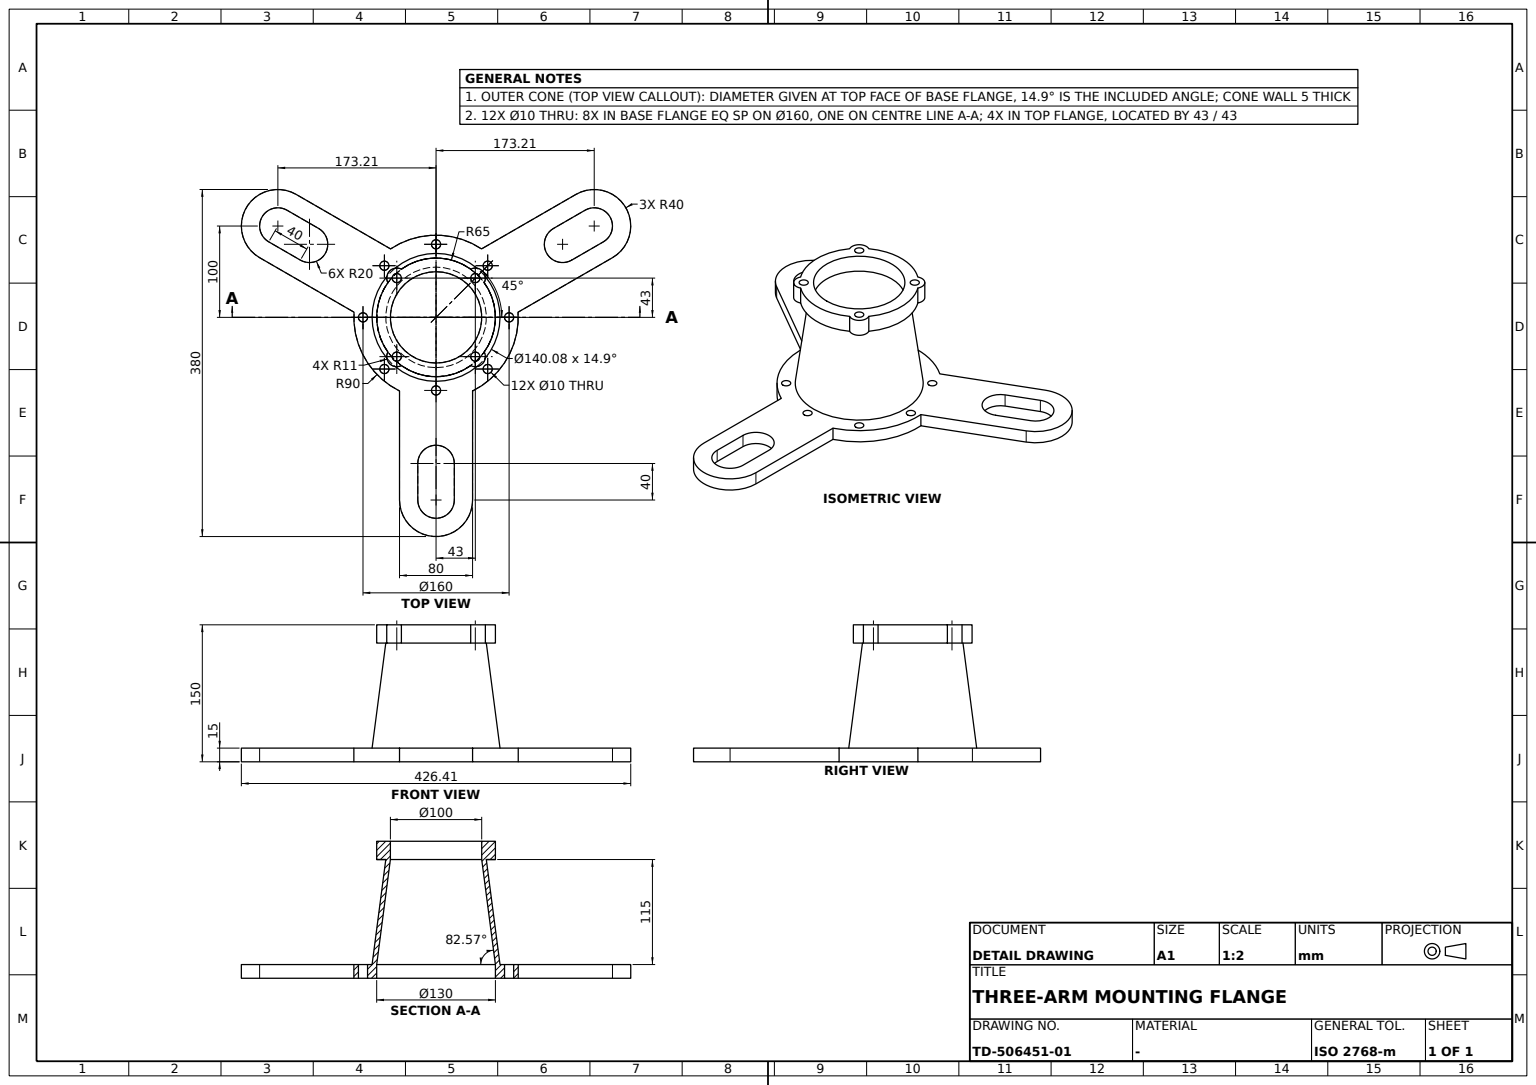
CATIA V5 part; units mm, degrees
sketch "Sketch1" plane through (0, 0, 0) normal (0, 0, 1) x (1, 0, 0)
  point P0 (200, 0)
  arc A0 (80.6226, 40) -> (-5.6703, 89.8212) centre (0, 0) ccw
  point P1 (0, 90)
  arc A1 (200, -20) -> (200, 20) centre (200, 0) ccw
  arc A2 (160, 20) -> (160, -20) centre (160, 0) ccw
  point P2 (160, 0)
  line L0 (160, 20) -> (200, 20)
  point P3 (160, 20)
  point P4 (200, 20)
  line L1 (160, 0) -> (180, 0) construction
  point P5 (180, 0)
  point P6 (200, -20)
  point P7 (160, -20)
  line L2 (160, -20) -> (200, -20)
  point P8 (80.6226, 40)
  line L3 (80.6226, 40) -> (200, 40)
  point P9 (200, 40)
  point P10 (200, -40)
  point P11 (80.6226, -40)
  line L4 (80.6226, -40) -> (200, -40)
  arc A3 (200, -40) -> (200, 40) centre (200, 0) ccw
  point P12 (-100, 173.2051)
  point P13 (-80, 138.5641)
  point P14 (-97.3205, 128.5641)
  point P15 (-117.3205, 163.2051)
  point P16 (-90, 155.8846)
  line L5 (-80, 138.5641) -> (-90, 155.8846) construction
  point P17 (-82.6795, 183.2051)
  point P18 (-62.6795, 148.5641)
  point P19 (-74.9523, 49.8212)
  point P20 (-134.641, 153.2051)
  point P21 (-65.359, 193.2051)
  point P22 (-5.6703, 89.8212)
  arc A4 (-82.6795, 183.2051) -> (-117.3205, 163.2051) centre (-100, 173.2051) ccw
  arc A5 (-97.3205, 128.5641) -> (-62.6795, 148.5641) centre (-80, 138.5641) ccw
  line L6 (-97.3205, 128.5641) -> (-117.3205, 163.2051)
  line L7 (-62.6795, 148.5641) -> (-82.6795, 183.2051)
  line L8 (-74.9523, 49.8212) -> (-134.641, 153.2051)
  line L9 (-5.6703, 89.8212) -> (-65.359, 193.2051)
  arc A6 (-65.359, 193.2051) -> (-134.641, 153.2051) centre (-100, 173.2051) ccw
  point P23 (-100, -173.2051)
  point P24 (-80, -138.5641)
  point P25 (-62.6795, -148.5641)
  point P26 (-82.6795, -183.2051)
  point P27 (-90, -155.8846)
  line L10 (-80, -138.5641) -> (-90, -155.8846) construction
  point P28 (-117.3205, -163.2051)
  point P29 (-97.3205, -128.5641)
  point P30 (-5.6703, -89.8212)
  point P31 (-65.359, -193.2051)
  point P32 (-134.641, -153.2051)
  point P33 (-74.9523, -49.8212)
  arc A7 (-117.3205, -163.2051) -> (-82.6795, -183.2051) centre (-100, -173.2051) ccw
  arc A8 (-62.6795, -148.5641) -> (-97.3205, -128.5641) centre (-80, -138.5641) ccw
  line L11 (-62.6795, -148.5641) -> (-82.6795, -183.2051)
  line L12 (-97.3205, -128.5641) -> (-117.3205, -163.2051)
  line L13 (-5.6703, -89.8212) -> (-65.359, -193.2051)
  line L14 (-74.9523, -49.8212) -> (-134.641, -153.2051)
  arc A9 (-134.641, -153.2051) -> (-65.359, -193.2051) centre (-100, -173.2051) ccw
  arc A10 (-74.9523, 49.8212) -> (-74.9523, -49.8212) centre (0, 0) ccw
  arc A11 (-5.6703, -89.8212) -> (80.6226, -40) centre (0, 0) ccw
  circle A12 centre (0, 0) radius 80 construction
  point P34 (0, 0)
  circle A13 centre (80, 0) radius 5
  point P35 (80, 0)
  circle A14 centre (56.5685, -56.5685) radius 5
  circle A15 centre (0, -80) radius 5
  circle A16 centre (-56.5685, -56.5685) radius 5
  circle A17 centre (-80, 0) radius 5
  circle A18 centre (-56.5685, 56.5685) radius 5
  circle A19 centre (0, 80) radius 5
  circle A20 centre (56.5685, 56.5685) radius 5
  dimension "distance y axis P0" = 200
  dimension "radius A0" = 90
  dimension "radius A1" = 20
  dimension "distance P0 P2" = 40
  dimension "distance P12 P13" = 40
  dimension "radius A4" = 20
  dimension "radius A7" = 20
  dimension "distance P23 P24" = 40
  dimension "radius A12" = 80
  dimension "radius A13" = 5
  dimension "radius A14" = 5
  dimension "radius A15" = 5
  dimension "radius A16" = 5
  dimension "radius A17" = 5
  dimension "radius A18" = 5
  dimension "radius A19" = 5
  dimension "radius A20" = 5
  constraint coincidence P0 x-axis
  constraint coincidence A0 P1
  constraint coincidence P1 y-axis
  constraint coincidence P2 x-axis
  constraint coincidence P5 A2
  constraint coincidence P16 A5
  constraint coincidence P27 A8
  constraint coincidence A0 A10
  constraint coincidence A10 A11
  constraint coincidence P34 L10
  constraint coincidence P34 x-axis
  constraint coincidence P35 A12
  constraint coincidence P35 x-axis
  constraint horizontal L0 x-axis
  constraint horizontal L3 x-axis
  constraint tangency A2 L0
  constraint tangency L0 A1
  constraint tangency A5 L6
  constraint tangency L6 A4
  constraint tangency L11 A7
  constraint tangency A8 L11
  constraint symmetry P4 P6 L1
  constraint symmetry P3 P7 L1
  constraint symmetry L0 L2 L1
  constraint symmetry P9 P10 L1
  constraint symmetry P8 P11 L1
  constraint symmetry L3 L4 L1
  constraint symmetry P15 P17 L5
  constraint symmetry P14 P18 L5
  constraint symmetry L6 L7 L5
  constraint symmetry P20 P21 L5
  constraint symmetry P19 P22 L5
  constraint symmetry L8 L9 L5
  constraint symmetry P31 P32 L10
  constraint symmetry P30 P33 L10
  constraint symmetry L13 L14 L10
  constraint symmetry P26 P28 L10
  constraint symmetry P25 P29 L10
  constraint symmetry L11 L12 L10
extrude "Pad1" add sketch "Sketch1" along normal blind 15
sketch "Sketch2" plane through (0, 0, 0) normal (1, 0, 0) x (0, 1, 0)
  point P0 (-65, 15)
  line L0 (-65, 15) -> (-50, 130)
  point P1 (-50, 130)
  line L1 (-90, 15) -> (-40, 15) construction
  line L2 (-70.0424, 15) -> (-55.0424, 130)
  point P2 (-70.0424, 15)
  point P3 (-55.0424, 130)
  line L3 (-65, 15) -> (-70.0424, 15)
  point P4 (-70.0424, 15)
  line L4 (-90, 15) -> (-40, 15) construction
  point P5 (-50, 130)
  line L5 (-50, 130) -> (-55.0424, 130)
  point P6 (-55.0424, 130)
  line L6 (-90, 15) -> (-40, 15) construction
  dimension "distance y axis P0" = 65
  dimension "distance y axis P1" = 50
  dimension "distance L0 L2" = 5
  dimension "distance L6 P3" = 115
  constraint coincidence L1 P0
  constraint coincidence P2 L4
  constraint coincidence P4 P2
  constraint coincidence P5 L0
  constraint coincidence P3 L5
  constraint coincidence P6 P3
  constraint coincidence P1 P5
  constraint horizontal L3 x-axis
  constraint horizontal L5 x-axis
revolve "Shaft1" add sketch "Sketch2" angle 360 about axis through (0, 0, 0) along (0, 0, 1)
sketch "Sketch3" plane through (0, 0, 15) normal (0, 0, 1) x (1, 0, 0)
  circle A0 centre (0, 0) radius 65
  point P0 (0, -65)
  dimension "radius A0" = 65
  constraint coincidence A0 P0
  constraint coincidence P0 y-axis
extrude "Pocket1" cut sketch "Sketch3" against normal blind 15
sketch "Sketch4" plane through (0, 0, 130) normal (0, 0, 1) x (1, 0, 0)
  arc A0 (37.9491, 52.7718) -> (-37.9491, 52.7718) centre (0, 0) ccw
  circle A1 centre (0, 0) radius 50
  point P0 (43, 43)
  line L0 (0, 0) -> (43, 43) construction
  circle A2 centre (43, 43) radius 5
  point P1 (43, 43)
  point P2 (37.9491, 52.7718)
  point P3 (34.0304, 36.6324)
  point P4 (36.6324, 34.0304)
  arc A3 (52.7718, 37.9491) -> (37.9491, 52.7718) centre (43, 43) ccw
  point P5 (52.7718, 37.9491)
  point P6 (-37.9491, 52.7718)
  point P7 (-52.7718, 37.9491)
  circle A4 centre (-43, 43) radius 5
  arc A5 (-52.7718, 37.9491) -> (-37.9491, 52.7718) centre (-43, 43) cw
  point P8 (37.9491, -52.7718)
  point P9 (52.7718, -37.9491)
  point P10 (-37.9491, -52.7718)
  point P11 (-52.7718, -37.9491)
  circle A6 centre (43, -43) radius 5
  arc A7 (52.7718, -37.9491) -> (37.9491, -52.7718) centre (43, -43) cw
  circle A8 centre (-43, -43) radius 5
  arc A9 (-52.7718, -37.9491) -> (-37.9491, -52.7718) centre (-43, -43) ccw
  arc A10 (-52.7718, 37.9491) -> (-52.7718, -37.9491) centre (0, 0) ccw
  arc A11 (-37.9491, -52.7718) -> (37.9491, -52.7718) centre (0, 0) ccw
  arc A12 (52.7718, -37.9491) -> (52.7718, 37.9491) centre (0, 0) ccw
  dimension "radius A0" = 65
  dimension "radius A1" = 50
  dimension "angle L0 x axis" = 45
  dimension "distance y axis P0" = 43
  dimension "radius A2" = 5
  constraint coincidence P1 L0
  constraint coincidence P1 P0
  constraint coincidence A1 P3
  constraint coincidence A1 P4
  constraint coincidence A0 A10
  constraint coincidence A11 A12
  constraint symmetry P2 P6 y-axis
  constraint symmetry P5 P7 y-axis
  constraint symmetry A2 A4 y-axis
  constraint symmetry A3 A5 y-axis
  constraint symmetry P2 P8 x-axis
  constraint symmetry P5 P9 x-axis
  constraint symmetry P6 P10 x-axis
  constraint symmetry P7 P11 x-axis
  constraint symmetry A2 A6 x-axis
  constraint symmetry A3 A7 x-axis
  constraint symmetry A4 A8 x-axis
  constraint symmetry A5 A9 x-axis
extrude "Pad2" add sketch "Sketch4" along normal blind 20
